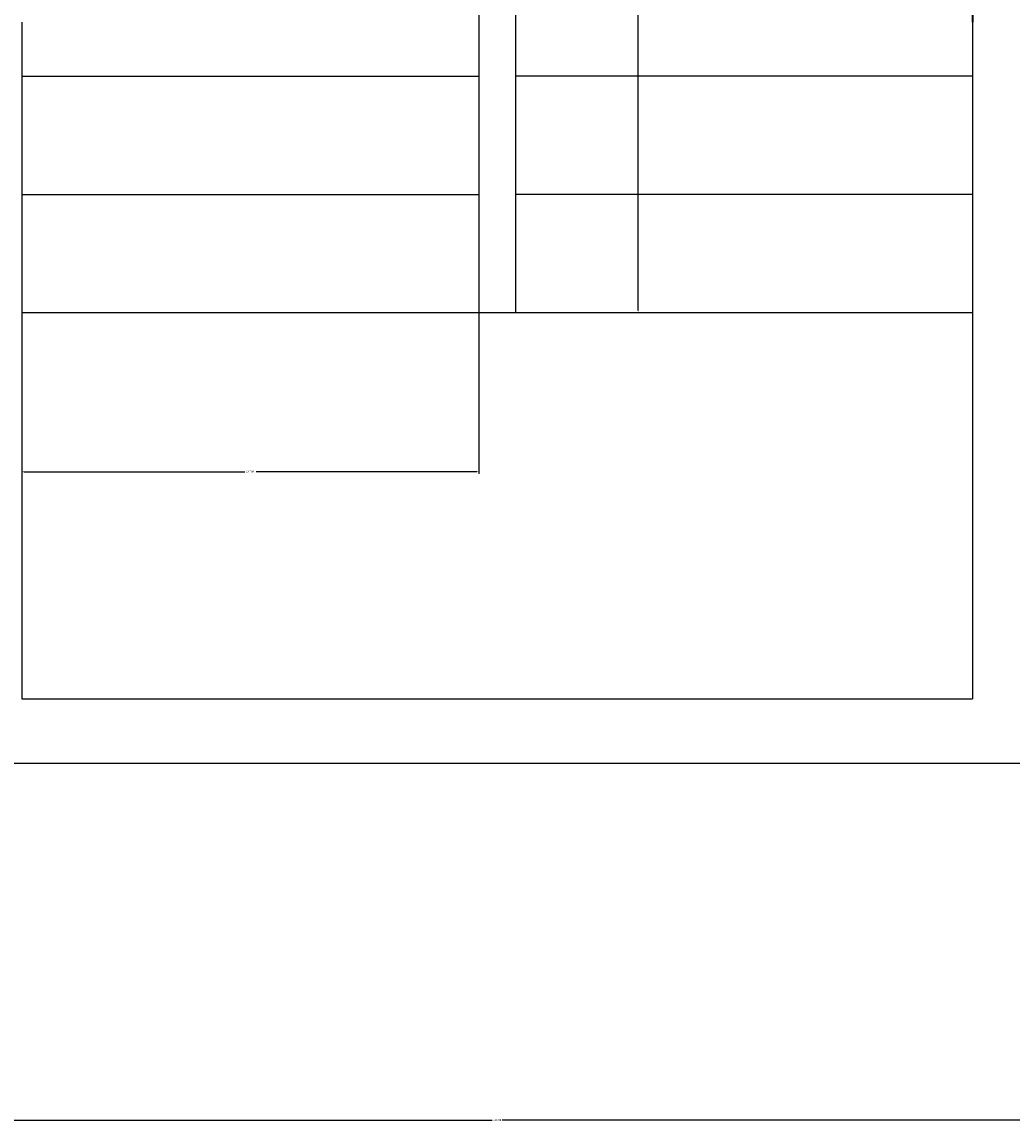
# Model space of a CAD drawing. Units: inches. Extents: x 4159 to 4826, y 299 to 1026.
# Tile 27 of 37: x 4453 to 4546, y 299 to 401. Entities that reach past the tile are written whole.
import ezdxf

# ---------------------------------------------------------------- set-up
doc = ezdxf.new("R2010")
doc.units = ezdxf.units.IN
for name, color, linetype, lineweight in [('A-ANNO-DIMS', 2, 'Continuous', 18), ('A-FLOR-STRS', 3, 'Continuous', 25), ('A-WALL', 7, 'Continuous', 35)]:
    doc.layers.add(name, color=color, linetype=linetype, lineweight=lineweight)
doc.styles.get("Standard").update_dxf_attribs({"font": 'arial.ttf'})
doc.dimstyles.get("Standard").update_dxf_attribs({"dimtxt": 0.18, "dimasz": 0.18, "dimexe": 0.18, "dimexo": 0.0625, "dimgap": 0.09, "dimtad": 0, "dimtih": 1, "dimtoh": 1, "dimdec": 4, "dimzin": 0, "dimdsep": 46, "dimtxsty": 'Standard', "dimcen": 0.09, "dimadec": 0, "dimazin": 0, "dimtfac": 1, "dimtdec": 4, "dimtofl": 0, "dimtmove": 0, "dimatfit": 3, "dimfxl": 1, "dimtolj": 1, "dimtzin": 0, "dimarcsym": 0})

# ---------------------------------------------------------------- blocks, each defined once
blk = doc.blocks.new('STAIR-FLIGHT-9-TREAD')
for p, q in [((0, 99), (42.58, 99)), ((42.58, 99), (42.58, 0)), ((0, 88), (42.58, 88)), ((0, 77), (42.58, 77)), ((0, 66), (42.58, 66)), ((0, 55), (42.58, 55)), ((0, 44), (42.58, 44)), ((0, 33), (42.58, 33)), ((0, 22), (42.58, 22)), ((0, 11), (42.58, 11))]:
    blk.add_line(p, q)
blk = doc.blocks.new('*D41')
at = {"layer": 'A-ANNO-DIMS', "color": 0, "lineweight": -2, "transparency": 16777216}
for p, q in [((4495.95, 473.2), (4510.92, 473.2)), ((4510.74, 473.02), (4510.74, 423.88)), ((4510.74, 374.38), (4510.74, 423.51)), ((4495.95, 374.2), (4510.92, 374.2))]:
    blk.add_line(p, q, dxfattribs=at)
at = {"layer": 'A-ANNO-DIMS', "color": 0, "transparency": 16777216}
for points in [[(4510.71, 473.02), (4510.77, 473.02), (4510.74, 473.2)], [(4510.71, 374.38), (4510.77, 374.38), (4510.74, 374.2)]]:
    blk.add_solid(points, dxfattribs=at)
at = {"layer": 'Defpoints', "color": 0, "transparency": 16777216}
for p in [(4495.89, 473.2), (4510.74, 473.2), (4495.89, 374.2)]:
    blk.add_point(p, dxfattribs=at)
at = {"layer": 'A-ANNO-DIMS', "color": 0, "transparency": 16777216, "insert": (4510.74, 423.7), "char_height": 0.18, "attachment_point": 5}
blk.add_mtext('\\A1;STAIR FLIGHT 99 TYP.', dxfattribs=at)
blk = doc.blocks.new('*D42')
at = {"layer": 'A-ANNO-DIMS', "color": 0, "lineweight": -2, "transparency": 16777216}
for p, q in [((4453.31, 374.13), (4453.31, 359.17)), ((4495.89, 374.13), (4495.89, 359.17)), ((4453.49, 359.35), (4474.07, 359.35)), ((4495.71, 359.35), (4475.13, 359.35))]:
    blk.add_line(p, q, dxfattribs=at)
at = {"layer": 'A-ANNO-DIMS', "color": 0, "transparency": 16777216}
for points in [[(4453.49, 359.38), (4453.49, 359.32), (4453.31, 359.35)], [(4495.71, 359.38), (4495.71, 359.32), (4495.89, 359.35)]]:
    blk.add_solid(points, dxfattribs=at)
at = {"layer": 'Defpoints', "color": 0, "transparency": 16777216}
for p in [(4453.31, 374.2), (4495.89, 374.2), (4495.89, 359.35)]:
    blk.add_point(p, dxfattribs=at)
at = {"layer": 'A-ANNO-DIMS', "color": 0, "transparency": 16777216, "insert": (4474.6, 359.35), "char_height": 0.18, "attachment_point": 5}
blk.add_mtext('\\A1;43 TYP.', dxfattribs=at)
blk = doc.blocks.new('*D47')
at = {"layer": 'A-ANNO-DIMS', "color": 0, "lineweight": -2, "transparency": 16777216}
for p, q in [((4447.31, 332.13), (4447.31, 298.77)), ((4547.89, 332.13), (4547.89, 298.77)), ((4447.49, 298.95), (4497.14, 298.95)), ((4547.71, 298.95), (4498.06, 298.95))]:
    blk.add_line(p, q, dxfattribs=at)
at = {"layer": 'A-ANNO-DIMS', "color": 0, "transparency": 16777216}
for points in [[(4447.49, 298.98), (4447.49, 298.92), (4447.31, 298.95)], [(4547.71, 298.98), (4547.71, 298.92), (4547.89, 298.95)]]:
    blk.add_solid(points, dxfattribs=at)
at = {"layer": 'Defpoints', "color": 0, "transparency": 16777216}
for p in [(4447.31, 332.2), (4547.89, 332.2), (4547.89, 298.95)]:
    blk.add_point(p, dxfattribs=at)
at = {"layer": 'A-ANNO-DIMS', "color": 0, "transparency": 16777216, "insert": (4497.6, 298.95), "char_height": 0.18, "attachment_point": 5}
blk.add_mtext('\\A1;100.58', dxfattribs=at)

msp = doc.modelspace()

# ---------------------------------------------------------------- linework, layer by layer
at = {"layer": 'A-FLOR-STRS'}
for p, q in [((4453.31, 401.254), (4453.31, 392.254)), ((4541.889, 401.254), (4541.889, 392.254)), ((4453.31, 392.254), (4453.31, 338.195)), ((4541.889, 392.254), (4541.889, 338.195)), ((4453.31, 374.195), (4541.889, 374.195)), ((4453.31, 338.195), (4541.889, 338.195)), ((4447.31, 332.195), (4547.889, 332.195))]:
    msp.add_line(p, q, dxfattribs=at)
at = {"layer": 'A-WALL'}
msp.add_line((4541.889, 618.254), (4541.889, 401.254), dxfattribs=at)

# ---------------------------------------------------------------- block references
at = {"layer": 'A-FLOR-STRS'}
msp.add_blockref('STAIR-FLIGHT-9-TREAD', (4453.31, 374.195), dxfattribs=at)
at = {"layer": 'A-FLOR-STRS', "extrusion": (0, 0, -1), "zscale": -1}
msp.add_blockref('STAIR-FLIGHT-9-TREAD', (-4541.889, 374.195), dxfattribs=at)

# ---------------------------------------------------------------- dimensions: what is measured, and where the dimension line sits
at = {"layer": 'A-ANNO-DIMS'}
dim = msp.add_linear_dim(base=(4510.739, 473.195), p1=(4495.889, 374.195), p2=(4495.889, 473.195), angle=90, text='STAIR FLIGHT <> TYP.', dimstyle='Standard', override={"dimdec": 0, "dimlfac": 1, "dimrnd": 0, "dimzin": 0, "dimdsep": 46, "dimlunit": 2}, dxfattribs=at)
dim.commit()
dim.dimension.update_dxf_attribs({"geometry": '*D41', "text_midpoint": (4510.739, 423.695)})
dim = msp.add_linear_dim(base=(4495.889, 359.345), p1=(4453.31, 374.195), p2=(4495.889, 374.195), text='<> TYP.', dimstyle='Standard', override={"dimdec": 0, "dimlfac": 1, "dimrnd": 0, "dimzin": 0, "dimdsep": 46, "dimlunit": 2}, dxfattribs=at)
dim.commit()
dim.dimension.update_dxf_attribs({"geometry": '*D42', "text_midpoint": (4474.6, 359.345)})
dim = msp.add_linear_dim(base=(4547.889, 298.945), p1=(4447.31, 332.195), p2=(4547.889, 332.195), dimstyle='Standard', override={"dimdec": 2, "dimlfac": 1, "dimrnd": 0, "dimzin": 0, "dimdsep": 46, "dimlunit": 2}, dxfattribs=at)
dim.commit()
dim.dimension.update_dxf_attribs({"geometry": '*D47', "text_midpoint": (4497.6, 298.945)})

doc.saveas('drawing.dxf')
